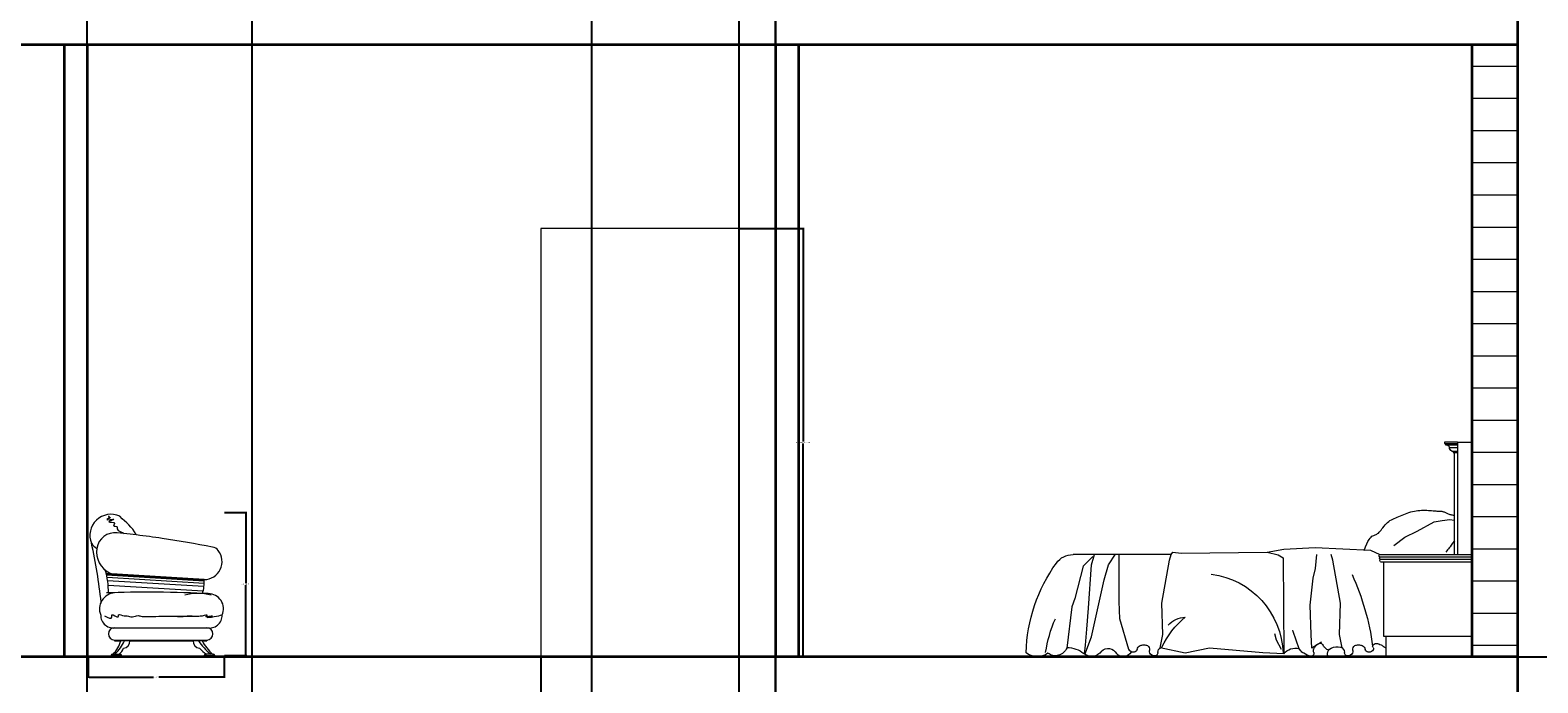
# Model space of a CAD drawing. Units: inches. Extents: x 1355 to 2746, y 1171 to 2751.
# Tile 22 of 24: x 2215 to 2510, y 2346 to 2474. Entities that reach past the tile are written whole.
import ezdxf

# ---------------------------------------------------------------- set-up
doc = ezdxf.new("R2010")
doc.units = ezdxf.units.IN
for name, color, linetype, lineweight in [('A-ANNO-DIMS', 2, 'Continuous', 18), ('A-FURN', 8, 'Continuous', 13), ('A-SECT', 7, 'Continuous', 35), ('A-SECT-DOOR', 3, 'Continuous', 18), ('A-WALL-PATT', 252, 'Continuous', 13)]:
    doc.layers.add(name, color=color, linetype=linetype, lineweight=lineweight)
doc.styles.get("Standard").update_dxf_attribs({"font": 'arial.ttf'})
doc.dimstyles.get("Standard").update_dxf_attribs({"dimtxt": 0.18, "dimasz": 0.18, "dimexe": 0.18, "dimexo": 0.0625, "dimgap": 0.09, "dimtad": 0, "dimtih": 1, "dimtoh": 1, "dimdec": 4, "dimzin": 0, "dimdsep": 46, "dimtxsty": 'Standard', "dimcen": 0.09, "dimadec": 0, "dimazin": 0, "dimtfac": 1, "dimtdec": 4, "dimtofl": 0, "dimtmove": 0, "dimatfit": 3, "dimfxl": 1, "dimtolj": 1, "dimtzin": 0, "dimarcsym": 0})

# ---------------------------------------------------------------- blocks, each defined once
blk = doc.blocks.new('A$C2FF713C3')
for p, q in [((0, 1050.5), (0, 0.5)), ((70, 1050.5), (0, 1050.5)), ((70, 1050.5), (70, 500.5)), ((70, 1050.5), (133.7, 1050.5)), ((127.4, 1044.2), (70, 1044.2)), ((125.8, 1038), (70, 1038)), ((127.4, 1038), (125.8, 1038)), ((133.7, 1044.2), (127.4, 1044.2)), ((127.4, 1044.2), (127.4, 1038)), ((133.7, 1050.5), (133.7, 1044.2)), ((108.5, 1024.2), (70, 1024.2)), ((91.3, 1006.7), (70, 1006.7)), ((91.3, 1000.5), (70, 1000.5)), ((85, 1000.5), (85, 500.5)), ((97.5, 1006.7), (91.3, 1006.7)), ((91.3, 1006.7), (91.3, 1000.5)), ((87.4, 693.2), (83.6, 693.1)), ((107.4, 672.2), (85.3, 669.2)), ((91.2, 693.6), (87.4, 693.2)), ((95.1, 694.2), (91.2, 693.6)), ((99, 694.9), (95.1, 694.2)), ((102.9, 695.9), (99, 694.9)), ((106.8, 697), (102.9, 695.9)), ((110.7, 698.3), (106.8, 697)), ((144.4, 667.7), (107.4, 672.2)), ((114.5, 699.7), (110.7, 698.3)), ((118.2, 701.2), (114.5, 699.7)), ((121.8, 702.9), (118.2, 701.2)), ((125.3, 704.5), (121.8, 702.9)), ((128.7, 706.1), (125.3, 704.5)), ((131.9, 707.6), (128.7, 706.1)), ((134.9, 709), (131.9, 707.6)), ((137.8, 710.2), (134.9, 709)), ((140.5, 711.1), (137.8, 710.2)), ((143, 711.8), (140.5, 711.1)), ((145.5, 712.2), (143, 711.8)), ((184.4, 660.3), (144.4, 667.7)), ((148, 712.5), (145.5, 712.2)), ((150.6, 712.6), (148, 712.5)), ((153.6, 712.7), (150.6, 712.6)), ((156.9, 712.7), (153.6, 712.7)), ((160.7, 712.8), (156.9, 712.7)), ((165.1, 713), (160.7, 712.8)), ((170.2, 713.4), (165.1, 713)), ((175.9, 713.9), (170.2, 713.4)), ((182.3, 714.4), (175.9, 713.9)), ((189.2, 715), (182.3, 714.4)), ((196.5, 715.6), (189.2, 715)), ((204.1, 716.2), (196.5, 715.6)), ((212.1, 716.7), (204.1, 716.2)), ((220.3, 717.1), (212.1, 716.7)), ((228.7, 717.3), (220.3, 717.1)), ((237.2, 717.3), (228.7, 717.3)), ((245.8, 717.1), (237.2, 717.3)), ((254.4, 716.7), (245.8, 717.1)), ((263.2, 715.9), (254.4, 716.7)), ((271.9, 714.8), (263.2, 715.9)), ((280.7, 713.3), (271.9, 714.8)), ((289.5, 711.4), (280.7, 713.3)), ((298.2, 709.1), (289.5, 711.4)), ((306.9, 706.4), (298.2, 709.1)), ((315.5, 703.4), (306.9, 706.4)), ((324, 700.1), (315.5, 703.4)), ((332.3, 696.8), (324, 700.1)), ((340.6, 693.4), (332.3, 696.8)), ((348.7, 690), (340.6, 693.4)), ((356.6, 686.7), (348.7, 690)), ((364.3, 683.5), (356.6, 686.7)), ((371.9, 680.4), (364.3, 683.5)), ((379.2, 677.3), (371.9, 680.4)), ((386.3, 674), (379.2, 677.3)), ((393.1, 670.5), (386.3, 674)), ((399.8, 666.5), (393.1, 670.5)), ((406.2, 662.1), (399.8, 666.5)), ((267.2, 614.5), (184.4, 660.3)), ((327.9, 585), (267.2, 614.5)), ((412.3, 657), (406.2, 662.1)), ((418.1, 651.3), (412.3, 657)), ((423.7, 645.1), (418.1, 651.3)), ((429.1, 638.6), (423.7, 645.1)), ((434.2, 632), (429.1, 638.6)), ((439, 625.6), (434.2, 632)), ((443.7, 619.6), (439, 625.6)), ((448.1, 614.1), (443.7, 619.6)), ((452.4, 609.5), (448.1, 614.1)), ((456.4, 605.9), (452.4, 609.5)), ((460.3, 603), (456.4, 605.9)), ((464.2, 600.8), (460.3, 603)), ((468, 599.1), (464.2, 600.8)), ((471.7, 597.6), (468, 599.1)), ((475.6, 596.1), (471.7, 597.6)), ((479.6, 594.4), (475.6, 596.1)), ((483.7, 592.3), (479.6, 594.4)), ((488, 589.7), (483.7, 592.3)), ((84.9, 568), (93.7, 555.7)), ((93.7, 555.7), (100.6, 546.3)), ((100.6, 546.3), (105.9, 539)), ((105.9, 539), (110.1, 533.2)), ((110.1, 533.2), (113.9, 528.2)), ((113.9, 528.2), (117.6, 523.3)), ((117.6, 523.3), (121.8, 517.9)), ((121.8, 517.9), (127, 511.4)), ((381.3, 544.7), (327.9, 585)), ((495.7, 521.8), (450, 500.5)), ((492.6, 586), (488, 589.7)), ((497.4, 581), (492.6, 586)), ((766.6, 534.5), (495.7, 521.8)), ((502.4, 574.2), (497.4, 581)), ((507.8, 565.1), (502.4, 574.2)), ((513.4, 553.5), (507.8, 565.1)), ((519.3, 538.8), (513.4, 553.5)), ((525.6, 520.7), (519.3, 538.8)), ((919.2, 526), (766.6, 534.5)), ((1001, 512.1), (919.2, 526)), ((450, 500.5), (0, 500.5)), ((450, 488.5), (0, 488.5)), ((448.7, 477.5), (0, 477.5)), ((446.9, 465.5), (0, 465.5)), ((431.9, 465.5), (431.9, 100.5)), ((642.6, 263.3), (679.4, 472.9)), ((679.4, 472.9), (687.3, 500.5)), ((764.1, 432.4), (757.6, 500.5)), ((923, 485), (919.8, 13.9)), ((947.7, 499.8), (923, 485)), ((1001, 512.1), (947.7, 499.8)), ((1422.2, 508), (1001, 512.1)), ((1463.2, 511.6), (1422.2, 508)), ((1471.1, 500.5), (1463.2, 511.6)), ((1479, 472.9), (1471.1, 500.5)), ((1471.1, 500.5), (1951, 500.5)), ((1515.8, 263.3), (1479, 472.9)), ((1725.7, 369.9), (1725.7, 500.5)), ((1776.6, 450.8), (1743.5, 502.3)), ((1798.7, 377.3), (1776.6, 450.8)), ((1861.3, 450.8), (1846, 500.5)), ((1853.9, 491.3), (1901.8, 443.5)), ((1876, 237.5), (1861.3, 450.8)), ((1901.8, 443.5), (1942.3, 285.3)), ((775.1, 384.6), (764.1, 432.4)), ((789.8, 252.2), (775.1, 384.6)), ((1725.7, 270.6), (1725.7, 369.9)), ((1861.3, 97.8), (1798.7, 377.3)), ((646.3, 108.8), (642.6, 263.3)), ((786.1, 108.8), (789.8, 252.2)), ((1512.2, 108.8), (1515.8, 263.3)), ((1722, 186), (1725.7, 270.6)), ((1883.4, 134.6), (1876, 237.5)), ((1942.3, 285.3), (1957, 244.9)), ((1957, 244.9), (1981.3, 42.2)), ((1677.5, 36.3), (1722, 186)), ((431.9, 100.5), (0, 100.5)), ((419.9, 100.5), (419.9, 0.5)), ((634, 43.7), (646.3, 108.8)), ((782.5, 42.6), (786.1, 108.8)), ((844.9, 39.6), (874.4, 124.2)), ((874.4, 124.2), (875.1, 130)), ((956.4, 83.1), (931.8, 36.9)), ((964.4, 113.4), (956.4, 83.1)), ((1524.4, 43.7), (1512.2, 108.8)), ((1892.4, 12.1), (1861.3, 97.8)), ((1890.7, 57.3), (1883.4, 134.6)), ((0, 0.5), (419.9, 0.5)), ((734.6, 72), (782.5, 42.6)), ((919.8, 13.9), (1021.5, 19.4)), ((1021.5, 19.4), (1282.6, 41.6)), ((1282.6, 41.6), (1401.6, 17.8)), ((1401.6, 17.8), (1524.4, 43.7)), ((1894.7, 13.8), (1890.7, 57.3))]:
    blk.add_line(p, q)
for centre, radius, start, end in [((125, 1021.3), 16.8, 87.42116, 169.92904), ((90, 1023.7), 18.5, 293.7928, 1.50079), ((435.7, 473.3), 13.6, 324.97742, 17.95445), ((443.2, 483.7), 8.28, 310.99411, 35.0512), ((447.3, 494.5), 6.6, 294.61118, 65.38882), ((1951, 400.5), 100, 35.83195, 90), ((1396.7, 0.2), 783.8, 1.45705, 35.83195), ((1735.3, -117.1), 1261.8, 155.69024, 172.29016), ((1327.7, 3.6), 404.9, 97.57237, 178.02017), ((1400.1, 81.1), 112.5, 40.70885, 88.9264), ((1125.8, -139.2), 432.6, 25.56932, 50.29378), ((1449, -72.7), 642.9, 8.37443, 23.73381), ((259.9, 249), 261.9, 307.63119, 310.56693), ((478.1, -13.1), 79.2, 115.93806, 127.15402), ((517.4, -93.9), 169, 111.78143, 115.93806), ((474.5, 13.6), 53.3, 104.37799, 111.78143), ((466.1, 46.3), 19.5, 71.58245, 104.37799), ((464.6, 41.9), 24.2, 42.22901, 71.58245), ((490.7, 39.5), 10.2, 140.3102, 217.27929), ((475.7, 51.9), 9.23, 320.3102, 42.22901), ((513.6, 57), 39, 217.27929, 233.1579), ((500.7, 39.8), 17.5, 233.1579, 256.94088), ((500.6, 39.4), 17.2, 256.94088, 270), ((500.6, 74), 51.8, 270, 277.51528), ((505.3, 38.6), 16, 277.51528, 349.78267), ((546.4, 31.2), 25.7, 114.29273, 169.78267), ((554.4, 13.4), 45.2, 90, 114.29273), ((554.4, 20.7), 37.9, 63.42724, 90), ((562.2, 36.4), 20.3, 346.09021, 63.42724), ((601.7, 26.6), 20.3, 166.09021, 243.58133), ((609.7, 42.8), 38.3, 243.58133, 251.5824), ((612.4, 50.9), 46.9, 251.5824, 258.81111), ((606.5, 21.1), 16.5, 258.81111, 1.75785), ((648.9, 22.4), 25.9, 104.59371, 181.75785), ((658.8, -15.6), 65.2, 63.45814, 104.59371), ((673, 12.8), 33.4, 4.66977, 63.45814), ((674.1, 83.9), 58.7, 296.89415, 314.45228), ((713.3, 7.3), 7.4, 170.64836, 198.63453), ((677.4, 13.2), 29, 350.64836, 4.66977), ((711.6, 6.7), 5.58, 198.63453, 218.42959), ((207.6, 559.5), 724.9, 314.45228, 314.97091), ((575.9, 190.8), 203.8, 314.97091, 315.94905), ((696.8, 73.9), 35.6, 315.94905, 329.81727), ((762.4, 35.7), 40.4, 136.79901, 149.81727), ((740.9, 55.9), 10.9, 81.87802, 136.79901), ((738.1, 36.1), 30.8, 50.07733, 81.87802), ((735.6, 33.1), 34.7, 33.71681, 50.07733), ((690, 2.7), 89.5, 23.5428, 33.71681), ((747.6, 27.8), 26.6, 343.69737, 23.5428), ((788.5, 15.9), 15.9, 163.69737, 216.05798), ((783.9, 12.5), 10.2, 216.05798, 282.98191), ((759.3, 118.9), 119.4, 282.98191, 301.5385), ((783.2, 80.1), 73.8, 301.5385, 318.3377), ((782.8, 80.4), 74.3, 318.3377, 326.7067), ((863.8, -27), 69.2, 36.67542, 105.79154), ((957.7, 57), 57.3, 227.99499, 228.65775), ((1509.5, 22.4), 25.9, 358.24215, 61.16814), ((1551.9, 21.1), 16.5, 178.24215, 281.18889), ((1546, 50.9), 46.9, 281.18889, 288.4176), ((1548.7, 42.8), 38.3, 288.4176, 296.41867), ((1556.8, 26.6), 20.3, 296.41867, 13.90979), ((1596.2, 36.4), 20.3, 116.57276, 193.90979), ((1604, 20.7), 37.9, 90, 116.57276), ((1604, 13.4), 45.2, 65.70727, 90), ((1612, 31.2), 25.7, 10.21733, 65.70727), ((1653.1, 38.6), 16, 190.21733, 262.48472), ((1657.8, 74), 51.8, 262.48472, 270), ((1657.8, 39.4), 17.2, 270, 283.05912), ((1657.7, 39.8), 17.5, 283.05912, 306.8421), ((1704.6, 43.4), 43.5, 208.05971, 320.53056), ((1644.8, 57), 39, 306.8421, 322.72071), ((1667.7, 39.5), 10.2, 322.72071, 344.91412), ((1779.5, -6.4), 46.9, 46.72075, 151.78128), ((1859.7, 59.2), 57.3, 213.23769, 312.00501), ((1983.6, -94.9), 140.5, 91.35454, 127.50961), ((2036.9, 65.4), 60.1, 201.78863, 308.33048), ((2126, 84.9), 84.4, 232.07783, 309.92484)]:
    blk.add_arc(centre, radius, start, end)
blk = doc.blocks.new('A$C28ED0BDC')
for p, q in [((300.7, 778.6), (176.5, 792.9)), ((737.6, 490.8), (105.1, 529.1)), ((737.6, 485.8), (106.3, 524)), ((737.6, 480.8), (107.5, 518.9)), ((737.5, 465.8), (110.8, 503.7)), ((735.8, 445.9), (114.2, 483.5)), ((730.6, 416.3), (117.6, 453.3)), ((158.9, 100), (753.7, 100)), ((158.9, 100), (158.9, 95)), ((169.3, 180), (753.7, 180)), ((753.7, 100), (753.7, 95)), ((204.4, 0), (136.7, 0)), ((151.7, 10), (146, 10)), ((151.7, 10), (189.4, 10)), ((158.9, 95), (200.3, 95)), ((195, 10), (189.4, 10)), ((195, 10), (189.4, 10)), ((257.3, 95), (200.3, 95)), ((257.3, 95), (666.7, 95)), ((723.7, 95), (666.7, 95)), ((723.7, 95), (753.7, 95)), ((737.8, 0), (805.4, 0)), ((747.1, 10), (752.8, 10)), ((747.1, 10), (752.8, 10)), ((790.4, 10), (752.8, 10)), ((790.4, 10), (796.1, 10))]:
    blk.add_line(p, q)
for centre, radius, start, end in [((135.3, 776.3), 135.9, 65.3492, 202.21563), ((162.8, 673.6), 120, 83.43842, 170.98936), ((-3552.4, -58.3), 3647.1, 6.37823, 12.40155), ((93.2, 779.5), 99.8, 213.09621, 240.68048), ((193.2, 668.8), 150.8, 170.98936, 243.39142), ((780.2, 642.1), 60, 37.32442, 79.59851), ((737, 606.7), 115.8, 270.2622, 38.33495), ((-328, 418.8), 446.9, 358.17507, 17.23744), ((179.4, 641.3), 120, 243.39142, 252.67687), ((458.5, 479.3), 279.3, 343.50497, 2.36848), ((164.5, 301.2), 103.1, 93.095, 202.35798), ((696.5, 85.3), 315.8, 74.36238, 105.63762), ((763.8, 301.7), 98.3, 336.20857, 89.98148), ((151.5, 260.4), 82.4, 178.89673, 282.44534), ((771.4, 260.4), 82.4, 257.55466, 1.10327), ((158.9, 140), 40, 90, 270), ((753.7, 140), 40, 270, 90), ((148.9, -2), 12.3, 103.33506, 170.71519), ((-63.8, 189.5), 280.5, 320.20721, 340.30535), ((-29.3, 210.6), 277.5, 313.71744, 335.39036), ((124.1, 86.8), 100.8, 310.34673, 337.03101), ((192.2, -2), 12.3, 9.28481, 76.66494), ((210.9, 93.5), 46.4, 277.43329, 1.84553), ((713.1, 93.5), 46.4, 178.15447, 262.56671), ((987.3, 281.2), 341.5, 213.0378, 232.56776), ((831, 152.1), 162.1, 220.15958, 241.18286), ((1022.2, 260.8), 341.5, 209.04881, 227.25949), ((750, -2), 12.3, 103.33506, 170.71519), ((793.3, -2), 12.3, 9.28481, 76.66494)]:
    blk.add_arc(centre, radius, start, end)
for points, knots in [([(123.9, 901.3), (120.7, 897.9), (113.5, 890.1), (146.7, 895.3), (73.3, 866.1), (197.2, 892.5), (86.1, 854.7), (175.1, 866.1), (141.9, 832.2), (182.3, 838), (163.3, 800.3), (225.2, 796.2), (219.8, 787.9)], [0, 0, 0, 0, 9.765075, 22.239713, 47.817951, 93.447543, 130.976544, 169.416587, 185.180341, 209.428428, 221.888603, 276.469797, 276.469797, 276.469797, 276.469797]), ([(300.7, 778.6), (300.1, 779.6), (269.8, 832.3), (237.8, 855.2), (192, 899.8)], [244.920573, 244.920573, 244.920573, 244.920573, 247.928636, 395.738949, 395.738949, 395.738949, 395.738949]), ([(791, 701.1), (682.8, 721), (519.9, 750.6), (355.8, 771.9), (300.7, 778.6)], [18.761969, 18.761969, 18.761969, 18.761969, 348.756072, 515.290542, 515.290542, 515.290542, 515.290542]), ([(763.8, 400), (674.2, 404.2), (398.1, 413.1), (207.8, 407.5), (107.2, 404.2)], [0, 0, 0, 0, 269.198238, 571.026582, 571.026582, 571.026582, 571.026582]), ([(93.5, 256.7), (117.3, 244.2), (148.3, 227.9), (135.5, 280.6), (184.2, 233.2), (182.4, 277.4), (213.7, 254), (239, 258.5), (267.4, 245.2), (313.7, 262.9), (325.5, 247.1), (418.5, 255), (547.8, 252.8), (616.1, 255.7), (660.2, 256.5)], [0, 0, 0, 0, 49.407579, 64.565784, 105.844847, 118.345477, 155.269185, 167.410003, 198.361737, 241.285001, 308.128282, 447.747709, 520.592639, 652.828768, 652.828768, 652.828768, 652.828768]), ([(848.7, 261.5), (836.7, 257.2), (814, 248.9), (727, 241.4), (826.7, 263.1), (729.9, 243.1), (771.4, 265.6), (713.2, 252.2), (686.6, 252.2), (629, 252.7), (589.5, 250.5), (564.7, 249.2)], [0, 0, 0, 0, 49.380651, 92.855981, 126.791693, 168.915675, 179.762432, 213.696461, 251.182, 296.320949, 372.653556, 372.653556, 372.653556, 372.653556])]:
    blk.add_open_spline(points, degree=3, knots=knots)
blk = doc.blocks.new('DOOR-OPENING-SECTION')
for p, q in [((0, 84), (0, 0)), ((38.81, 84), (0, 84)), ((38.81, 84), (38.81, 0))]:
    blk.add_line(p, q)
blk = doc.blocks.new('*D91')
at = {"layer": 'A-ANNO-DIMS', "color": 0, "lineweight": -2, "transparency": 16777216}
for p, q in [((2252.87, 2379.65), (2257.19, 2379.65)), ((2257.01, 2379.47), (2257.01, 2365.82)), ((2257.01, 2351.8), (2257.01, 2365.45)), ((2252.87, 2351.62), (2257.19, 2351.62))]:
    blk.add_line(p, q, dxfattribs=at)
at = {"layer": 'A-ANNO-DIMS', "color": 0, "transparency": 16777216}
for points in [[(2256.98, 2379.47), (2257.04, 2379.47), (2257.01, 2379.65)], [(2256.98, 2351.8), (2257.04, 2351.8), (2257.01, 2351.62)]]:
    blk.add_solid(points, dxfattribs=at)
at = {"layer": 'Defpoints', "color": 0, "transparency": 16777216}
for p in [(2252.8, 2379.65), (2257.01, 2379.65), (2252.8, 2351.62)]:
    blk.add_point(p, dxfattribs=at)
at = {"layer": 'A-ANNO-DIMS', "color": 0, "transparency": 16777216, "insert": (2257.01, 2365.64), "char_height": 0.18, "attachment_point": 5}
blk.add_mtext('\\A1;CHAIR 28 TYP.', dxfattribs=at)
blk = doc.blocks.new('*D92')
at = {"layer": 'A-ANNO-DIMS', "color": 0, "lineweight": -2, "transparency": 16777216}
for p, q in [((2226.12, 2351.56), (2226.12, 2347.24)), ((2252.8, 2351.56), (2252.8, 2347.24)), ((2226.3, 2347.42), (2238.93, 2347.42)), ((2252.62, 2347.42), (2239.99, 2347.42))]:
    blk.add_line(p, q, dxfattribs=at)
at = {"layer": 'A-ANNO-DIMS', "color": 0, "transparency": 16777216}
for points in [[(2226.3, 2347.45), (2226.3, 2347.39), (2226.12, 2347.42)], [(2252.62, 2347.45), (2252.62, 2347.39), (2252.8, 2347.42)]]:
    blk.add_solid(points, dxfattribs=at)
at = {"layer": 'Defpoints', "color": 0, "transparency": 16777216}
for p in [(2226.12, 2351.62), (2252.8, 2351.62), (2252.8, 2347.42)]:
    blk.add_point(p, dxfattribs=at)
at = {"layer": 'A-ANNO-DIMS', "color": 0, "transparency": 16777216, "insert": (2239.46, 2347.42), "char_height": 0.18, "attachment_point": 5}
blk.add_mtext('\\A1;27 TYP.', dxfattribs=at)
blk = doc.blocks.new('*D93')
at = {"layer": 'A-ANNO-DIMS', "color": 0, "lineweight": -2, "transparency": 16777216}
for p, q in [((2353.77, 2435.4), (2366.49, 2435.4)), ((2366.31, 2435.22), (2366.31, 2393.58)), ((2366.31, 2351.58), (2366.31, 2393.22)), ((2353.77, 2351.4), (2366.49, 2351.4))]:
    blk.add_line(p, q, dxfattribs=at)
at = {"layer": 'A-ANNO-DIMS', "color": 0, "transparency": 16777216}
for points in [[(2366.28, 2435.22), (2366.34, 2435.22), (2366.31, 2435.4)], [(2366.28, 2351.58), (2366.34, 2351.58), (2366.31, 2351.4)]]:
    blk.add_solid(points, dxfattribs=at)
at = {"layer": 'Defpoints', "color": 0, "transparency": 16777216}
for p in [(2353.71, 2435.4), (2366.31, 2435.4), (2353.71, 2351.4)]:
    blk.add_point(p, dxfattribs=at)
at = {"layer": 'A-ANNO-DIMS', "color": 0, "transparency": 16777216, "insert": (2366.31, 2393.4), "char_height": 0.18, "attachment_point": 5}
blk.add_mtext('\\A1;DOOR OPENING 84 TYP.', dxfattribs=at)
blk = doc.blocks.new('*D94')
at = {"layer": 'A-ANNO-DIMS', "color": 0, "lineweight": -2, "transparency": 16777216}
for p, q in [((2314.9, 2351.34), (2314.9, 2338.62)), ((2353.71, 2351.34), (2353.71, 2338.62)), ((2315.08, 2338.8), (2333.78, 2338.8)), ((2353.53, 2338.8), (2334.83, 2338.8))]:
    blk.add_line(p, q, dxfattribs=at)
at = {"layer": 'A-ANNO-DIMS', "color": 0, "transparency": 16777216}
for points in [[(2315.08, 2338.83), (2315.08, 2338.77), (2314.9, 2338.8)], [(2353.53, 2338.83), (2353.53, 2338.77), (2353.71, 2338.8)]]:
    blk.add_solid(points, dxfattribs=at)
at = {"layer": 'Defpoints', "color": 0, "transparency": 16777216}
for p in [(2314.9, 2351.4), (2353.71, 2351.4), (2353.71, 2338.8)]:
    blk.add_point(p, dxfattribs=at)
at = {"layer": 'A-ANNO-DIMS', "color": 0, "transparency": 16777216, "insert": (2334.31, 2338.8), "char_height": 0.18, "attachment_point": 5}
blk.add_mtext('\\A1;39 TYP.', dxfattribs=at)
blk = doc.blocks.new('*D99')
at = {"layer": 'A-ANNO-DIMS', "color": 0, "lineweight": -2, "transparency": 16777216}
for p, q in [((2080.39, 2139.36), (2080.39, 2716.58)), ((2080.57, 2716.4), (2152.75, 2716.4)), ((2225.71, 2716.4), (2153.53, 2716.4)), ((2225.89, 2139.36), (2225.89, 2716.58))]:
    blk.add_line(p, q, dxfattribs=at)
at = {"layer": 'A-ANNO-DIMS', "color": 0, "transparency": 16777216}
for points in [[(2080.57, 2716.43), (2080.57, 2716.37), (2080.39, 2716.4)], [(2225.71, 2716.43), (2225.71, 2716.37), (2225.89, 2716.4)]]:
    blk.add_solid(points, dxfattribs=at)
at = {"layer": 'Defpoints', "color": 0, "transparency": 16777216}
for p in [(2225.89, 2716.4), (2080.39, 2139.3), (2225.89, 2139.3)]:
    blk.add_point(p, dxfattribs=at)
at = {"layer": 'A-ANNO-DIMS', "color": 0, "transparency": 16777216, "insert": (2153.14, 2716.4), "char_height": 0.18, "attachment_point": 5}
blk.add_mtext('\\A1;145.5', dxfattribs=at)
blk = doc.blocks.new('*D100')
at = {"layer": 'A-ANNO-DIMS', "color": 0, "lineweight": -2, "transparency": 16777216}
for p, q in [((2225.89, 2139.36), (2225.89, 2716.58)), ((2226.07, 2716.4), (2293.11, 2716.4)), ((2360.71, 2716.4), (2293.67, 2716.4)), ((2360.89, 2139.36), (2360.89, 2716.58))]:
    blk.add_line(p, q, dxfattribs=at)
at = {"layer": 'A-ANNO-DIMS', "color": 0, "transparency": 16777216}
for points in [[(2226.07, 2716.43), (2226.07, 2716.37), (2225.89, 2716.4)], [(2360.71, 2716.43), (2360.71, 2716.37), (2360.89, 2716.4)]]:
    blk.add_solid(points, dxfattribs=at)
at = {"layer": 'Defpoints', "color": 0, "transparency": 16777216}
for p in [(2360.89, 2716.4), (2225.89, 2139.3), (2360.89, 2139.3)]:
    blk.add_point(p, dxfattribs=at)
at = {"layer": 'A-ANNO-DIMS', "color": 0, "transparency": 16777216, "insert": (2293.39, 2716.4), "char_height": 0.18, "attachment_point": 5}
blk.add_mtext('\\A1;135', dxfattribs=at)
blk = doc.blocks.new('*D101')
at = {"layer": 'A-ANNO-DIMS', "color": 0, "lineweight": -2, "transparency": 16777216}
for p, q in [((2360.89, 2139.36), (2360.89, 2716.58)), ((2361.07, 2716.4), (2433.25, 2716.4)), ((2506.21, 2716.4), (2434.03, 2716.4)), ((2506.39, 2139.36), (2506.39, 2716.58))]:
    blk.add_line(p, q, dxfattribs=at)
at = {"layer": 'A-ANNO-DIMS', "color": 0, "transparency": 16777216}
for points in [[(2361.07, 2716.43), (2361.07, 2716.37), (2360.89, 2716.4)], [(2506.21, 2716.43), (2506.21, 2716.37), (2506.39, 2716.4)]]:
    blk.add_solid(points, dxfattribs=at)
at = {"layer": 'Defpoints', "color": 0, "transparency": 16777216}
for p in [(2506.39, 2716.4), (2360.89, 2139.3), (2506.39, 2139.3)]:
    blk.add_point(p, dxfattribs=at)
at = {"layer": 'A-ANNO-DIMS', "color": 0, "transparency": 16777216, "insert": (2433.64, 2716.4), "char_height": 0.18, "attachment_point": 5}
blk.add_mtext('\\A1;145.5', dxfattribs=at)
blk = doc.blocks.new('*D112')
at = {"layer": 'A-ANNO-DIMS', "color": 0, "lineweight": -2, "transparency": 16777216}
for p, q in [((2258.27, 2095.29), (2258.27, 2716.58)), ((2258.45, 2716.4), (2291.19, 2716.4)), ((2324.72, 2716.4), (2291.98, 2716.4)), ((2324.9, 2095.29), (2324.9, 2716.58))]:
    blk.add_line(p, q, dxfattribs=at)
at = {"layer": 'A-ANNO-DIMS', "color": 0, "transparency": 16777216}
for points in [[(2258.45, 2716.43), (2258.45, 2716.37), (2258.27, 2716.4)], [(2324.72, 2716.43), (2324.72, 2716.37), (2324.9, 2716.4)]]:
    blk.add_solid(points, dxfattribs=at)
at = {"layer": 'Defpoints', "color": 0, "transparency": 16777216}
for p in [(2324.9, 2716.4), (2258.27, 2095.22), (2324.9, 2095.22)]:
    blk.add_point(p, dxfattribs=at)
at = {"layer": 'A-ANNO-DIMS', "color": 0, "transparency": 16777216, "insert": (2291.58, 2716.4), "char_height": 0.18, "attachment_point": 5}
blk.add_mtext('\\A1;66.63', dxfattribs=at)
blk = doc.blocks.new('*D116')
at = {"layer": 'A-ANNO-DIMS', "color": 0, "lineweight": -2, "transparency": 16777216}
for p, q in [((1976.77, 2477.4), (2648.07, 2477.4)), ((2647.89, 2477.22), (2647.89, 2414.58)), ((2647.89, 2351.58), (2647.89, 2414.22)), ((1976.77, 2351.4), (2648.07, 2351.4))]:
    blk.add_line(p, q, dxfattribs=at)
at = {"layer": 'A-ANNO-DIMS', "color": 0, "transparency": 16777216}
for points in [[(2647.86, 2477.22), (2647.92, 2477.22), (2647.89, 2477.4)], [(2647.86, 2351.58), (2647.92, 2351.58), (2647.89, 2351.4)]]:
    blk.add_solid(points, dxfattribs=at)
at = {"layer": 'Defpoints', "color": 0, "transparency": 16777216}
for p in [(1976.71, 2477.4), (2647.89, 2477.4), (1976.71, 2351.4)]:
    blk.add_point(p, dxfattribs=at)
at = {"layer": 'A-ANNO-DIMS', "color": 0, "transparency": 16777216, "insert": (2647.89, 2414.4), "char_height": 0.18, "attachment_point": 5}
blk.add_mtext('\\A1;126', dxfattribs=at)
blk = doc.blocks.new('*D128')
at = {"layer": 'A-ANNO-DIMS', "color": 0, "lineweight": -2, "transparency": 16777216}
for p, q in [((2506.45, 2477.4), (2648.07, 2477.4)), ((2647.89, 2477.22), (2647.89, 2414.58)), ((2647.89, 2351.58), (2647.89, 2414.22)), ((2506.45, 2351.4), (2648.07, 2351.4))]:
    blk.add_line(p, q, dxfattribs=at)
at = {"layer": 'A-ANNO-DIMS', "color": 0, "transparency": 16777216}
for points in [[(2647.86, 2477.22), (2647.92, 2477.22), (2647.89, 2477.4)], [(2647.86, 2351.58), (2647.92, 2351.58), (2647.89, 2351.4)]]:
    blk.add_solid(points, dxfattribs=at)
at = {"layer": 'Defpoints', "color": 0, "transparency": 16777216}
for p in [(2506.39, 2477.4), (2647.89, 2477.4), (2506.39, 2351.4)]:
    blk.add_point(p, dxfattribs=at)
at = {"layer": 'A-ANNO-DIMS', "color": 0, "transparency": 16777216, "insert": (2647.89, 2414.4), "char_height": 0.18, "attachment_point": 5}
blk.add_mtext('\\A1;126', dxfattribs=at)
blk = doc.blocks.new('*D134')
at = {"layer": 'A-ANNO-DIMS', "color": 0, "lineweight": -2, "transparency": 16777216}
for p, q in [((2353.71, 2477.34), (2353.71, 1171.06)), ((2360.89, 2477.34), (2360.89, 1171.06)), ((2353.89, 1171.24), (2356.92, 1171.24)), ((2360.71, 1171.24), (2357.68, 1171.24))]:
    blk.add_line(p, q, dxfattribs=at)
at = {"layer": 'A-ANNO-DIMS', "color": 0, "transparency": 16777216}
for points in [[(2353.89, 1171.27), (2353.89, 1171.21), (2353.71, 1171.24)], [(2360.71, 1171.27), (2360.71, 1171.21), (2360.89, 1171.24)]]:
    blk.add_solid(points, dxfattribs=at)
at = {"layer": 'Defpoints', "color": 0, "transparency": 16777216}
for p in [(2353.71, 2477.4), (2360.89, 2477.4), (2360.89, 1171.24)]:
    blk.add_point(p, dxfattribs=at)
at = {"layer": 'A-ANNO-DIMS', "color": 0, "transparency": 16777216, "insert": (2357.3, 1171.24), "char_height": 0.18, "attachment_point": 5}
blk.add_mtext('\\A1;7.181', dxfattribs=at)

msp = doc.modelspace()

# ---------------------------------------------------------------- hatches: boundary and pattern name
at = {"layer": 'A-WALL-PATT'}
h = msp.add_hatch(dxfattribs=at)
h.set_pattern_fill('ANSI31', color=256, scale=1.9874, angle=-45, style=0)
h.paths.add_polyline_path([(2497.3909, 2351.3999), (2506.3909, 2351.3999), (2506.3909, 2471.3999), (2497.3909, 2471.3999)])

# ---------------------------------------------------------------- linework, layer by layer
at = {"layer": 'A-SECT'}
for p, q in [((2506.3909, 2645.3999), (2506.3909, 2471.3999)), ((2506.3909, 2519.3999), (2506.3909, 2345.3999)), ((2506.3909, 2471.3999), (2080.3909, 2471.3999)), ((2221.3909, 2471.3999), (2221.3909, 2351.3999)), ((2225.8909, 2471.3999), (2225.8909, 2351.3999)), ((2360.8909, 2471.3999), (2360.8909, 2351.3999)), ((2365.3909, 2471.3999), (2365.3909, 2351.3999)), ((2497.3909, 2471.3999), (2497.3909, 2351.3999)), ((2506.3909, 2393.3999), (2506.3909, 2219.3999)), ((2506.3909, 2351.3999), (2080.3909, 2351.3999))]:
    msp.add_line(p, q, dxfattribs=at)

# ---------------------------------------------------------------- block references
at = {"layer": 'A-FURN'}
for name, p, xscale, yscale, zscale in [('A$C2FF713C3', (2497.3909, 2351.3801), -0.0400677785412672, 0.0400677785412672, 0.0400677785412672), ('A$C28ED0BDC', (2226.4664, 2351.6202), 0.0303702499100781, 0.0303702499100781, 0.0303702499100781)]:
    msp.add_blockref(name, p, dxfattribs=dict(at, xscale=xscale, yscale=yscale, zscale=zscale))
at = {"layer": 'A-SECT-DOOR'}
msp.add_blockref('DOOR-OPENING-SECTION', (2314.902, 2351.4), dxfattribs=at)

# ---------------------------------------------------------------- dimensions: what is measured, and where the dimension line sits
at = {"layer": 'A-ANNO-DIMS'}
for base, p1, p2, override, picture, middle in [((2225.8909, 2716.3999), (2080.3909, 2139.3018), (2225.8909, 2139.3018), {"dimdec": 1, "dimlfac": 1, "dimrnd": 0, "dimzin": 0, "dimdsep": 46, "dimlunit": 2}, '*D99', (2153.1409, 2716.3999)), ((2360.8909, 2716.3999), (2225.8909, 2139.3018), (2360.8909, 2139.3018), {"dimdec": 0, "dimlfac": 1, "dimrnd": 0, "dimzin": 0, "dimdsep": 46, "dimlunit": 2}, '*D100', (2293.3909, 2716.3999)), ((2324.8959, 2716.3999), (2258.2658, 2095.2225), (2324.8959, 2095.2225), {"dimdec": 2, "dimlfac": 1, "dimrnd": 0, "dimzin": 0, "dimdsep": 46, "dimlunit": 2}, '*D112', (2291.5809, 2716.3999)), ((2506.3909, 2716.3999), (2360.8909, 2139.3018), (2506.3909, 2139.3018), {"dimdec": 1, "dimlfac": 1, "dimrnd": 0, "dimzin": 0, "dimdsep": 46, "dimlunit": 2}, '*D101', (2433.6409, 2716.3999)), ((2360.8909, 1171.2388), (2353.71, 2477.3999), (2360.8909, 2477.3999), {"dimdec": 3, "dimlfac": 1, "dimrnd": 0, "dimzin": 0, "dimdsep": 46, "dimlunit": 2}, '*D134', (2357.3004, 1171.2388))]:
    dim = msp.add_linear_dim(base=base, p1=p1, p2=p2, dimstyle='Standard', override=override, dxfattribs=at)
    dim.commit()
    dim.dimension.update_dxf_attribs({"geometry": picture, "text_midpoint": middle})
for p1, p2, picture in [((1976.7083, 2351.3999), (1976.7083, 2477.3999), '*D116'), ((2506.3909, 2351.3999), (2506.3909, 2477.3999), '*D128')]:
    dim = msp.add_linear_dim(base=(2647.886, 2477.3999), p1=p1, p2=p2, angle=90, dimstyle='Standard', override={"dimdec": 0, "dimlfac": 1, "dimrnd": 0, "dimzin": 0, "dimdsep": 46, "dimlunit": 2}, dxfattribs=at)
    dim.commit()
    dim.dimension.update_dxf_attribs({"geometry": picture, "text_midpoint": (2647.886, 2414.3999)})
for base, p1, p2, text, picture, middle in [((2366.31, 2435.3999), (2353.71, 2351.3999), (2353.71, 2435.3999), 'DOOR OPENING <> TYP.', '*D93', (2366.31, 2393.3999)), ((2257.0079, 2379.6549), (2252.8027, 2351.6202), (2252.8027, 2379.6549), 'CHAIR <> TYP.', '*D91', (2257.0079, 2365.6376))]:
    dim = msp.add_linear_dim(base=base, p1=p1, p2=p2, angle=90, text=text, dimstyle='Standard', override={"dimdec": 0, "dimlfac": 1, "dimrnd": 0, "dimzin": 0, "dimdsep": 46, "dimlunit": 2}, dxfattribs=at)
    dim.commit()
    dim.dimension.update_dxf_attribs({"geometry": picture, "text_midpoint": middle})
for base, p1, p2, picture, middle in [((2252.8027, 2347.4151), (2226.116, 2351.6202), (2252.8027, 2351.6202), '*D92', (2239.4594, 2347.4151)), ((2353.71, 2338.7999), (2314.9023, 2351.3999), (2353.71, 2351.3999), '*D94', (2334.3062, 2338.7999))]:
    dim = msp.add_linear_dim(base=base, p1=p1, p2=p2, text='<> TYP.', dimstyle='Standard', override={"dimdec": 0, "dimlfac": 1, "dimrnd": 0, "dimzin": 0, "dimdsep": 46, "dimlunit": 2}, dxfattribs=at)
    dim.commit()
    dim.dimension.update_dxf_attribs({"geometry": picture, "text_midpoint": middle})

doc.saveas('drawing.dxf')
